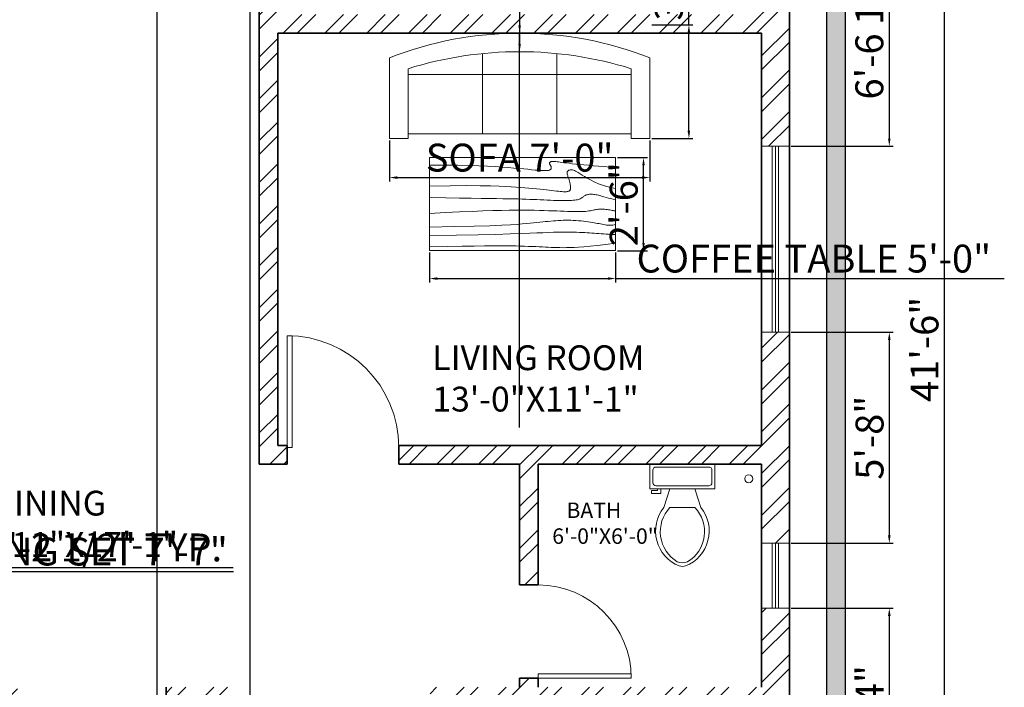
# Model space of a CAD drawing. Units: inches. Extents: x 418 to 1041, y 2094 to 2761.
# Tile 4 of 5: x 723 to 1041, y 2308 to 2523. Entities that reach past the tile are written whole.
import ezdxf

# ---------------------------------------------------------------- set-up
doc = ezdxf.new("R2010")
doc.units = ezdxf.units.IN
for name, color, linetype, lineweight in [('A-ANNO-DIMS', 2, 'Continuous', 18), ('A-AREA-IDEN', 7, 'Continuous', 18), ('A-DOOR', 4, 'Continuous', 18), ('A-FLOR-FIXT', 9, 'Continuous', 18), ('A-FURN', 8, 'Continuous', 18), ('A-GLAZ', 244, 'Continuous', 18), ('A-WALL', 7, 'Continuous', 35), ('A-WALL-PATT', 252, 'Continuous', 13), ('L-WALL', 7, 'Continuous', 25), ('L-WALL-PATT', 252, 'Continuous', 13)]:
    doc.layers.add(name, color=color, linetype=linetype, lineweight=lineweight)
doc.styles.get("Standard").update_dxf_attribs({"font": 'arial.ttf'})
doc.dimstyles.new('ISO-25', dxfattribs={"dimtxt": 9, "dimasz": 2.5, "dimexe": 1.25, "dimexo": 0.625, "dimtad": 1, "dimlunit": 3, "dimtxsty": 'Standard', "dimcen": 2.5, "dimadec": 0, "dimazin": 0, "dimtfac": 1, "dimtmove": 0, "dimatfit": 3, "dimfxl": 1, "dimarcsym": 0})

# ---------------------------------------------------------------- blocks, each defined once
blk = doc.blocks.new('*U2')
for p, q in [((0, 0), (0, -6)), ((40, 0), (40, -6))]:
    blk.add_line(p, q)
blk.add_lwpolyline([(0, 0), (0, 40), (1.75, 40), (1.75, 0)], close=True)
blk.add_arc((0, 0), 40, 0, 90)
blk = doc.blocks.new('*U7')
for p, q in [((0, 0), (0, -6)), ((-40, 0), (-40, -6))]:
    blk.add_line(p, q)
blk.add_lwpolyline([(0, 0), (0, 40), (-1.75, 40), (-1.75, 0)], close=True)
blk.add_arc((0, 0), 40, 90, 180)
blk = doc.blocks.new('*U10')
for p, q in [((9.5, -6), (9.5, -2)), ((-10, -8.5), (-8, -8.5)), ((-10, -9.5), (-10, -8.5)), ((-7, -9.5), (-10, -9.5)), ((-8, -8.5), (-8, -8)), ((-7, -8), (-7, -9.5)), ((-4, -8), (-6, -14)), ((4, -8), (6, -14)), ((4, -14), (-4, -14))]:
    blk.add_line(p, q)
blk.add_lwpolyline([(10.5, -8), (10.5, 0), (-10.5, 0), (-10.5, -8)], close=True)
for points in [[(-9.5, -2), (-9.5, -6)], [(8.5, -1), (-8.5, -1)], [(-8.5, -7), (8.5, -7)]]:
    blk.add_lwpolyline(points)
for centre, radius, start, end in [((-8.62, -1.88), 0.884, 81.8699, 188.1301), ((8.62, -1.88), 0.884, 351.8699, 98.1301), ((-8.62, -6.12), 0.884, 171.8699, 278.1301), ((8.62, -6.12), 0.884, 261.8699, 8.1301), ((3.52, -21.58), 12.17, 141.4691, 247.9714), ((4.2, -21.82), 11.33, 136.3677, 238.9468), ((-3.52, -21.58), 12.17, 292.0284, 38.5307), ((-4.2, -21.82), 11.33, 301.053, 43.6321), ((0, -27.88), 4, 245.7318, 294.2682), ((0, -29), 4, 254.8605, 285.1395)]:
    blk.add_arc(centre, radius, start, end)
blk = doc.blocks.new('Sofa - Roundback 7 ft.')
for p, q in [((-12.00002, -32.4421), (-12.00003, -6.5971)), ((11.99997, -32.4421), (11.99998, -6.5971)), ((-36.000027, -34), (-36.000027, -11.4696)), ((35.99998, -34), (35.99998, -11.4696)), ((-35.999844, -13.3819), (35.9998, -13.3819)), ((-36.000027, -32.4421), (35.99998, -32.4421))]:
    blk.add_line(p, q)
for points in [[(-36.000027, -34), (-42.000027, -34), (-42.000027, -8)], [(41.99998, -8), (41.99998, -34), (35.99998, -34)]]:
    blk.add_lwpolyline(points)
for centre, radius, start, end in [((0, -114.25), 114.25, 68.43141, 111.5686), ((-0.00001, -127.1968), 121.1968, 72.72033, 107.2797)]:
    blk.add_arc(centre, radius, start, end)
blk = doc.blocks.new('Table - Rectangular Woodgrain 60 x 30 in.')
for p, q in [((0, 0), (0, -30)), ((60, 0), (0, 0)), ((60, -30), (60, 0)), ((0, -30), (60, -30))]:
    blk.add_line(p, q)
for points in [[(0, -2.4), (4.8155, -2.418), (9.0302, -2.4688), (12.709, -2.5477), (15.9167, -2.65), (18.7181, -2.7711), (21.1781, -2.9063), (23.3616, -3.0508), (25.3333, -3.2), (27.1477, -3.3495), (28.8172, -3.4958), (30.3437, -3.636), (31.7291, -3.7667), (32.9756, -3.8849), (34.0849, -3.9875), (35.059, -4.0714), (35.9, -4.1334), (36.6114, -4.1711), (37.2041, -4.1854), (37.6906, -4.1779), (38.0833, -4.15), (38.3948, -4.1034), (38.6375, -4.0396), (38.8239, -3.9602), (38.9666, -3.8667), (39.0764, -3.7608), (39.1573, -3.6448), (39.2116, -3.521), (39.2416, -3.3917), (39.2498, -3.2593), (39.2385, -3.1261), (39.21, -2.9944), (39.1666, -2.8667), (39.111, -2.7447), (39.0468, -2.6281), (38.978, -2.5163), (38.9083, -2.4083), (38.8418, -2.3035), (38.7823, -2.201), (38.7337, -2.1001), (38.7, -2), (38.6844, -1.9003), (38.6875, -1.8021), (38.7094, -1.707), (38.75, -1.6167), (38.8094, -1.5326), (38.8875, -1.4563), (38.9844, -1.3893), (39.1, -1.3333), (39.2351, -1.2896), (39.3937, -1.2583), (39.5804, -1.2396), (39.8, -1.2333), (40.057, -1.2396), (40.3562, -1.2583), (40.7023, -1.2896), (41.1, -1.3333), (41.5547, -1.3895), (42.0755, -1.4573), (42.6721, -1.5361), (43.3542, -1.625), (44.1316, -1.7233), (45.014, -1.8302), (46.0114, -1.9449), (47.1333, -2.0667), (48.3862, -2.1947), (49.7625, -2.3281), (51.2513, -2.4663), (52.8416, -2.6083), (54.5226, -2.7535), (56.2833, -2.9011), (58.1127, -3.0501), (60, -3.2)], [(0, -9.2), (6.5759, -9.0858), (11.9385, -9.0365), (16.2527, -9.0418), (19.6833, -9.0917), (22.3952, -9.1759), (24.5531, -9.2844), (26.322, -9.4069), (27.8666, -9.5333), (29.3241, -9.6553), (30.7203, -9.7719), (32.0532, -9.8837), (33.3208, -9.9917), (34.5213, -10.0965), (35.6526, -10.199), (36.7128, -10.2999), (37.7, -10.4), (38.6129, -10.4996), (39.4531, -10.5969), (40.223, -10.6895), (40.925, -10.775), (41.5613, -10.8512), (42.1344, -10.9156), (42.6465, -10.966), (43.1, -11), (43.4976, -11.0158), (43.8437, -11.0136), (44.143, -10.9942), (44.4, -10.9583), (44.6195, -10.9069), (44.8062, -10.8406), (44.9648, -10.7603), (45.1, -10.6667), (45.2155, -10.5598), (45.3114, -10.4365), (45.3871, -10.2929), (45.4416, -10.125), (45.4743, -9.929), (45.4844, -9.7011), (45.4709, -9.4371), (45.4333, -9.1333), (45.3716, -8.7883), (45.2896, -8.4104), (45.1919, -8.0107), (45.0833, -7.6), (44.9685, -7.1893), (44.8521, -6.7896), (44.7388, -6.4117), (44.6333, -6.0667), (44.54, -5.7628), (44.4614, -5.4979), (44.4001, -5.2675), (44.3583, -5.0667), (44.3384, -4.8909), (44.3427, -4.7354), (44.3736, -4.5956), (44.4333, -4.4667), (44.5236, -4.3453), (44.6427, -4.2333), (44.7884, -4.1339), (44.9583, -4.05), (45.1501, -3.9849), (45.3614, -3.9417), (45.59, -3.9234), (45.8333, -3.9333), (46.0915, -3.9749), (46.3734, -4.0531), (46.6906, -4.1736), (47.0542, -4.3417), (47.4756, -4.5629), (47.9661, -4.8427), (48.5372, -5.1866), (49.2, -5.6), (49.9676, -6.0844), (50.8594, -6.625), (51.8965, -7.2031), (53.1, -7.8), (54.491, -8.3969), (56.0906, -8.975), (57.9199, -9.5156), (60, -10)], [(0, -12.8), (5.1847, -12.9322), (9.6213, -13.0323), (13.3963, -13.1059), (16.5958, -13.1583), (19.3063, -13.1952), (21.614, -13.2219), (23.6054, -13.2439), (25.3666, -13.2667), (26.9728, -13.2947), (28.4531, -13.3281), (29.8256, -13.3663), (31.1083, -13.4083), (32.3191, -13.4535), (33.476, -13.501), (34.597, -13.5501), (35.7, -13.6), (36.7984, -13.6497), (37.8875, -13.6979), (38.9578, -13.743), (40, -13.7833), (41.0047, -13.8174), (41.9625, -13.8438), (42.864, -13.8607), (43.7, -13.8667), (44.4631, -13.8604), (45.1552, -13.8417), (45.7801, -13.8104), (46.3416, -13.7667), (46.8439, -13.7104), (47.2906, -13.6417), (47.6858, -13.5604), (48.0333, -13.4667), (48.3375, -13.3608), (48.6042, -13.2448), (48.8396, -13.121), (49.05, -12.9917), (49.2417, -12.8593), (49.4208, -12.7261), (49.5937, -12.5944), (49.7667, -12.4667), (49.9452, -12.3451), (50.1323, -12.2313), (50.3303, -12.1268), (50.5416, -12.0333), (50.7686, -11.9524), (51.0135, -11.8854), (51.2788, -11.8341), (51.5666, -11.8), (51.8785, -11.7843), (52.2116, -11.7865), (52.562, -11.8059), (52.926, -11.8417), (53.2998, -11.8931), (53.6795, -11.9594), (54.0614, -12.0397), (54.4416, -12.1333), (54.8223, -12.2401), (55.2293, -12.3625), (55.6942, -12.5037), (56.2489, -12.6667), (56.9251, -12.8547), (57.7545, -13.0708), (58.7689, -13.3182), (60, -13.6)], [(0, -18), (5.124, -17.7273), (9.6609, -17.5057), (13.6705, -17.3303), (17.2125, -17.1958), (20.3467, -17.0973), (23.1328, -17.0297), (25.6307, -16.9878), (27.9, -16.9667), (29.9928, -16.9617), (31.9302, -16.9703), (33.7254, -16.9907), (35.3917, -17.0208), (36.9423, -17.0588), (38.3906, -17.1026), (39.7499, -17.1503), (41.0333, -17.2), (42.2519, -17.2496), (43.4073, -17.2969), (44.4986, -17.3395), (45.525, -17.375), (46.4858, -17.4012), (47.3802, -17.4156), (48.2074, -17.416), (48.9667, -17.4), (49.6583, -17.3662), (50.2872, -17.3167), (50.8595, -17.2547), (51.3812, -17.1833), (51.8584, -17.1057), (52.2971, -17.025), (52.7034, -16.9443), (53.0833, -16.8667), (53.443, -16.7951), (53.789, -16.7313), (54.128, -16.6768), (54.4666, -16.6334), (54.8115, -16.6024), (55.1693, -16.5854), (55.5465, -16.5841), (55.95, -16.6), (56.3828, -16.6337), (56.8346, -16.6823), (57.2915, -16.7418), (57.7396, -16.8084), (58.165, -16.878), (58.5539, -16.9469), (58.8924, -17.0111), (59.1666, -17.0667), (59.3679, -17.1107), (59.5078, -17.1438), (59.6032, -17.1675), (59.6708, -17.1833), (59.7275, -17.193), (59.7901, -17.1979), (59.8753, -17.1998), (60, -17.2)], [(0, -22.4), (8.0098, -22.2501), (14.4094, -22.1011), (19.4168, -21.9535), (23.25, -21.8083), (26.1269, -21.6663), (28.2656, -21.5281), (29.884, -21.3947), (31.2, -21.2667), (32.3967, -21.1448), (33.5172, -21.0292), (34.5697, -20.9198), (35.5625, -20.8167), (36.5037, -20.7198), (37.4015, -20.6292), (38.2642, -20.5448), (39.1, -20.4667), (39.9164, -20.3951), (40.7187, -20.3313), (41.5117, -20.2768), (42.3, -20.2333), (43.0883, -20.2024), (43.8812, -20.1854), (44.6836, -20.1841), (45.5, -20.2), (46.3328, -20.234), (47.1747, -20.2844), (48.0163, -20.3488), (48.8479, -20.425), (49.66, -20.5106), (50.4429, -20.6031), (51.1872, -20.7004), (51.8833, -20.8), (52.5246, -20.8999), (53.1166, -20.9995), (53.6681, -21.0983), (54.1875, -21.1958), (54.6834, -21.2919), (55.1646, -21.3859), (55.6394, -21.4777), (56.1167, -21.5667), (56.6028, -21.6515), (57.0961, -21.7266), (57.5929, -21.7852), (58.0896, -21.8208), (58.5823, -21.8268), (59.0674, -21.7964), (59.5412, -21.723), (60, -21.6)], [(0, -25.2), (8.6355, -25.0504), (15.7026, -24.9031), (21.4049, -24.7606), (25.9458, -24.625), (29.529, -24.4988), (32.3578, -24.3844), (34.6359, -24.284), (36.5667, -24.2), (38.3213, -24.1341), (39.9417, -24.0854), (41.437, -24.0523), (42.8167, -24.0333), (44.0901, -24.0268), (45.2667, -24.0313), (46.3557, -24.0451), (47.3667, -24.0667), (48.309, -24.0947), (49.1928, -24.1287), (50.0284, -24.168), (50.826, -24.2125), (51.5959, -24.2617), (52.3483, -24.3151), (53.0935, -24.3725), (53.8417, -24.4334), (54.6009, -24.497), (55.3699, -24.561), (56.1454, -24.6226), (56.9239, -24.6792), (57.7021, -24.7279), (58.4764, -24.7662), (59.2435, -24.7911), (60, -24.8)], [(0, -28.8), (5.6867, -28.6681), (10.45, -28.5698), (14.407, -28.5012), (17.675, -28.4584), (20.3711, -28.4374), (22.6125, -28.4344), (24.5164, -28.4455), (26.2, -28.4667), (27.762, -28.4947), (29.2276, -28.5281), (30.6033, -28.5663), (31.8958, -28.6084), (33.1118, -28.6535), (34.2578, -28.7011), (35.3405, -28.7501), (36.3666, -28.8), (37.3443, -28.8497), (38.288, -28.8974), (39.2137, -28.9412), (40.1375, -28.9792), (41.0753, -29.0093), (42.0432, -29.0297), (43.0572, -29.0384), (44.1333, -29.0333), (45.2936, -29.0114), (46.5843, -28.9641), (48.0579, -28.8816), (49.7666, -28.7542), (51.7629, -28.5721), (54.0989, -28.3255), (56.8272, -28.0048), (60, -27.6)]]:
    blk.add_lwpolyline(points)
blk = doc.blocks.new('*D16')
at = {"layer": 'A-ANNO-DIMS', "color": 0, "lineweight": -2, "transparency": 16777216}
for p, q in [((972.18, 2666.03), (1022.79, 2666.03)), ((1021.54, 2663.53), (1021.54, 2170.53)), ((972.18, 2168.03), (1022.79, 2168.03))]:
    blk.add_line(p, q, dxfattribs=at)
at = {"layer": 'A-ANNO-DIMS', "color": 0, "transparency": 16777216}
for points in [[(1021.13, 2663.53), (1021.96, 2663.53), (1021.54, 2666.03)], [(1021.13, 2170.53), (1021.96, 2170.53), (1021.54, 2168.03)]]:
    blk.add_solid(points, dxfattribs=at)
at = {"layer": 'Defpoints', "color": 0, "transparency": 16777216}
for p in [(971.56, 2666.03), (971.56, 2168.03), (1021.54, 2168.03)]:
    blk.add_point(p, dxfattribs=at)
at = {"layer": 'A-ANNO-DIMS', "color": 0, "transparency": 16777216, "insert": (1016.32, 2417.03), "char_height": 9, "attachment_point": 5, "rotation": 90}
blk.add_mtext('41\'-6"', dxfattribs=at)
blk = doc.blocks.new('WIN-60IN')
for p, q in [((0, 5.5), (60, 5.5)), ((0, 4.5), (60, 4.5)), ((0, 3.5), (60, 3.5))]:
    blk.add_line(p, q)
blk.add_lwpolyline([(0, 9), (60, 9), (60, 0), (0, 0)], close=True)
blk = doc.blocks.new('WIN-21IN')
for p, q in [((0, 5.5), (21, 5.5)), ((0, 4.5), (21, 4.5)), ((0, 3.5), (21, 3.5))]:
    blk.add_line(p, q)
blk.add_lwpolyline([(0, 9), (21, 9), (21, 0), (0, 0)], close=True)
blk = doc.blocks.new('*D33')
at = {"layer": 'A-ANNO-DIMS', "color": 0, "lineweight": -2, "transparency": 16777216}
for p, q in [((638.78, 2346.93), (638.78, 2347.94)), ((641.34, 2346.93), (641.34, 2347.94)), ((636.28, 2346.69), (633.78, 2346.69)), ((638.78, 2346.69), (641.34, 2346.69)), ((643.84, 2346.69), (792.12, 2346.69))]:
    blk.add_line(p, q, dxfattribs=at)
at = {"layer": 'A-ANNO-DIMS', "color": 0, "transparency": 16777216}
for points in [[(636.28, 2347.11), (636.28, 2346.28), (638.78, 2346.69)], [(643.84, 2347.11), (643.84, 2346.28), (641.34, 2346.69)]]:
    blk.add_solid(points, dxfattribs=at)
at = {"layer": 'Defpoints', "color": 0, "transparency": 16777216}
for p in [(638.78, 2346.31), (641.34, 2346.69), (641.34, 2346.31)]:
    blk.add_point(p, dxfattribs=at)
at = {"layer": 'A-ANNO-DIMS', "color": 0, "transparency": 16777216, "insert": (719.23, 2351.97), "char_height": 9, "attachment_point": 5}
blk.add_mtext('RAIL POST 0\'-2 1/2" TYP.', dxfattribs=at)
blk = doc.blocks.new('*D35')
at = {"layer": 'A-ANNO-DIMS', "color": 0, "lineweight": -2, "transparency": 16777216}
for p, q in [((598.64, 2358.4), (598.64, 2344.13)), ((689.64, 2358.4), (689.64, 2344.13)), ((601.14, 2345.38), (687.14, 2345.38)), ((689.64, 2345.38), (792.31, 2345.38))]:
    blk.add_line(p, q, dxfattribs=at)
at = {"layer": 'A-ANNO-DIMS', "color": 0, "transparency": 16777216}
for points in [[(601.14, 2345.79), (601.14, 2344.96), (598.64, 2345.38)], [(687.14, 2345.79), (687.14, 2344.96), (689.64, 2345.38)]]:
    blk.add_solid(points, dxfattribs=at)
at = {"layer": 'Defpoints', "color": 0, "transparency": 16777216}
for p in [(598.64, 2359.03), (689.64, 2359.03), (689.64, 2345.38)]:
    blk.add_point(p, dxfattribs=at)
at = {"layer": 'A-ANNO-DIMS', "color": 0, "transparency": 16777216, "insert": (742.22, 2350.65), "char_height": 9, "attachment_point": 5}
blk.add_mtext('DINING SET 7\'-7"', dxfattribs=at)
blk = doc.blocks.new('*D37')
at = {"layer": 'A-ANNO-DIMS', "color": 0, "lineweight": -2, "transparency": 16777216}
for p, q in [((842.56, 2484.4), (842.56, 2471.18)), ((926.56, 2484.4), (926.56, 2471.18)), ((845.06, 2472.43), (924.06, 2472.43))]:
    blk.add_line(p, q, dxfattribs=at)
at = {"layer": 'A-ANNO-DIMS', "color": 0, "transparency": 16777216}
for points in [[(845.06, 2472.84), (845.06, 2472.01), (842.56, 2472.43)], [(924.06, 2472.84), (924.06, 2472.01), (926.56, 2472.43)]]:
    blk.add_solid(points, dxfattribs=at)
at = {"layer": 'Defpoints', "color": 0, "transparency": 16777216}
for p in [(842.56, 2485.03), (926.56, 2485.03), (926.56, 2472.43)]:
    blk.add_point(p, dxfattribs=at)
at = {"layer": 'A-ANNO-DIMS', "color": 0, "transparency": 16777216, "insert": (884.56, 2477.71), "char_height": 9, "attachment_point": 5}
blk.add_mtext('SOFA 7\'-0"', dxfattribs=at)
blk = doc.blocks.new('*D38')
at = {"layer": 'A-ANNO-DIMS', "color": 0, "lineweight": -2, "transparency": 16777216}
for p, q in [((939.16, 2521.69), (939.16, 2570.33)), ((927.18, 2521.69), (940.41, 2521.69)), ((939.16, 2487.53), (939.16, 2519.19)), ((927.18, 2485.03), (940.41, 2485.03))]:
    blk.add_line(p, q, dxfattribs=at)
at = {"layer": 'A-ANNO-DIMS', "color": 0, "transparency": 16777216}
for points in [[(938.74, 2519.19), (939.57, 2519.19), (939.16, 2521.69)], [(938.74, 2487.53), (939.57, 2487.53), (939.16, 2485.03)]]:
    blk.add_solid(points, dxfattribs=at)
at = {"layer": 'Defpoints', "color": 0, "transparency": 16777216}
for p in [(926.56, 2521.69), (939.16, 2521.69), (926.56, 2485.03)]:
    blk.add_point(p, dxfattribs=at)
at = {"layer": 'A-ANNO-DIMS', "color": 0, "transparency": 16777216, "insert": (933.88, 2547.26), "char_height": 9, "attachment_point": 5, "rotation": 90}
blk.add_mtext('3\'-0 1/2"', dxfattribs=at)
blk = doc.blocks.new('*D39')
at = {"layer": 'A-ANNO-DIMS', "color": 0, "lineweight": -2, "transparency": 16777216}
for p, q in [((855.52, 2448.24), (855.52, 2438.61)), ((915.52, 2448.24), (915.52, 2438.61)), ((858.02, 2439.86), (913.02, 2439.86)), ((915.52, 2439.86), (1040.9, 2439.86))]:
    blk.add_line(p, q, dxfattribs=at)
at = {"layer": 'A-ANNO-DIMS', "color": 0, "transparency": 16777216}
for points in [[(858.02, 2440.28), (858.02, 2439.44), (855.52, 2439.86)], [(913.02, 2440.28), (913.02, 2439.44), (915.52, 2439.86)]]:
    blk.add_solid(points, dxfattribs=at)
at = {"layer": 'Defpoints', "color": 0, "transparency": 16777216}
for p in [(855.52, 2448.86), (915.52, 2448.86), (915.52, 2439.86)]:
    blk.add_point(p, dxfattribs=at)
at = {"layer": 'A-ANNO-DIMS', "color": 0, "transparency": 16777216, "insert": (979.46, 2445.14), "char_height": 9, "attachment_point": 5}
blk.add_mtext('COFFEE TABLE 5\'-0"', dxfattribs=at)
blk = doc.blocks.new('*D40')
at = {"layer": 'A-ANNO-DIMS', "color": 0, "lineweight": -2, "transparency": 16777216}
for p, q in [((916.15, 2478.86), (925.77, 2478.86)), ((924.52, 2451.36), (924.52, 2476.36)), ((916.15, 2448.86), (925.77, 2448.86))]:
    blk.add_line(p, q, dxfattribs=at)
at = {"layer": 'A-ANNO-DIMS', "color": 0, "transparency": 16777216}
for points in [[(924.11, 2476.36), (924.94, 2476.36), (924.52, 2478.86)], [(924.11, 2451.36), (924.94, 2451.36), (924.52, 2448.86)]]:
    blk.add_solid(points, dxfattribs=at)
at = {"layer": 'Defpoints', "color": 0, "transparency": 16777216}
for p in [(915.52, 2478.86), (924.52, 2478.86), (915.52, 2448.86)]:
    blk.add_point(p, dxfattribs=at)
at = {"layer": 'A-ANNO-DIMS', "color": 0, "transparency": 16777216, "insert": (919.3, 2463.86), "char_height": 9, "attachment_point": 5, "rotation": 90}
blk.add_mtext('2\'-6"', dxfattribs=at)
blk = doc.blocks.new('*D48')
at = {"layer": 'A-ANNO-DIMS', "color": 0, "lineweight": -2, "transparency": 16777216}
for p, q in [((972.18, 2561.03), (1005.06, 2561.03)), ((1003.81, 2558.53), (1003.81, 2485.03)), ((972.18, 2482.53), (1005.06, 2482.53))]:
    blk.add_line(p, q, dxfattribs=at)
at = {"layer": 'A-ANNO-DIMS', "color": 0, "transparency": 16777216}
for points in [[(1003.39, 2558.53), (1004.22, 2558.53), (1003.81, 2561.03)], [(1003.39, 2485.03), (1004.22, 2485.03), (1003.81, 2482.53)]]:
    blk.add_solid(points, dxfattribs=at)
at = {"layer": 'Defpoints', "color": 0, "transparency": 16777216}
for p in [(971.56, 2561.03), (971.56, 2482.53), (1003.81, 2482.53)]:
    blk.add_point(p, dxfattribs=at)
at = {"layer": 'A-ANNO-DIMS', "color": 0, "transparency": 16777216, "insert": (998.53, 2521.78), "char_height": 9, "attachment_point": 5, "rotation": 90}
blk.add_mtext('6\'-6 1/2"', dxfattribs=at)
blk = doc.blocks.new('*D49')
at = {"layer": 'A-ANNO-DIMS', "color": 0, "lineweight": -2, "transparency": 16777216}
for p, q in [((972.18, 2422.53), (1005.06, 2422.53)), ((1003.81, 2420.03), (1003.81, 2357.03)), ((972.18, 2354.53), (1005.06, 2354.53))]:
    blk.add_line(p, q, dxfattribs=at)
at = {"layer": 'A-ANNO-DIMS', "color": 0, "transparency": 16777216}
for points in [[(1003.39, 2420.03), (1004.22, 2420.03), (1003.81, 2422.53)], [(1003.39, 2357.03), (1004.22, 2357.03), (1003.81, 2354.53)]]:
    blk.add_solid(points, dxfattribs=at)
at = {"layer": 'Defpoints', "color": 0, "transparency": 16777216}
for p in [(971.56, 2422.53), (971.56, 2354.53), (1003.81, 2354.53)]:
    blk.add_point(p, dxfattribs=at)
at = {"layer": 'A-ANNO-DIMS', "color": 0, "transparency": 16777216, "insert": (998.59, 2388.53), "char_height": 9, "attachment_point": 5, "rotation": 90}
blk.add_mtext('5\'-8"', dxfattribs=at)
blk = doc.blocks.new('*D50')
at = {"layer": 'A-ANNO-DIMS', "color": 0, "lineweight": -2, "transparency": 16777216}
for p, q in [((972.18, 2333.53), (1005.06, 2333.53)), ((1003.81, 2331.03), (1003.81, 2272.26)), ((972.18, 2269.76), (1005.06, 2269.76))]:
    blk.add_line(p, q, dxfattribs=at)
at = {"layer": 'A-ANNO-DIMS', "color": 0, "transparency": 16777216}
for points in [[(1003.39, 2331.03), (1004.22, 2331.03), (1003.81, 2333.53)], [(1003.39, 2272.26), (1004.22, 2272.26), (1003.81, 2269.76)]]:
    blk.add_solid(points, dxfattribs=at)
at = {"layer": 'Defpoints', "color": 0, "transparency": 16777216}
for p in [(971.56, 2333.53), (971.56, 2269.76), (1003.81, 2269.76)]:
    blk.add_point(p, dxfattribs=at)
at = {"layer": 'A-ANNO-DIMS', "color": 0, "transparency": 16777216, "insert": (998.61, 2301.64), "char_height": 9, "attachment_point": 5, "rotation": 90}
blk.add_mtext('5\'-4"', dxfattribs=at)
blk = doc.blocks.new('*D59')
at = {"layer": 'A-ANNO-DIMS', "color": 0, "lineweight": -2, "transparency": 16777216}
for p, q in [((767.56, 2582.4), (767.56, 2100.53)), ((797.56, 2582.4), (797.56, 2100.53)), ((770.06, 2101.78), (795.06, 2101.78))]:
    blk.add_line(p, q, dxfattribs=at)
at = {"layer": 'A-ANNO-DIMS', "color": 0, "transparency": 16777216}
for points in [[(770.06, 2102.19), (770.06, 2101.36), (767.56, 2101.78)], [(795.06, 2102.19), (795.06, 2101.36), (797.56, 2101.78)]]:
    blk.add_solid(points, dxfattribs=at)
at = {"layer": 'Defpoints', "color": 0, "transparency": 16777216}
for p in [(767.56, 2583.03), (797.56, 2583.03), (797.56, 2101.78)]:
    blk.add_point(p, dxfattribs=at)
at = {"layer": 'A-ANNO-DIMS', "color": 0, "transparency": 16777216, "insert": (782.56, 2107), "char_height": 9, "attachment_point": 5}
blk.add_mtext('2\'-6"', dxfattribs=at)
blk = doc.blocks.new('*D70')
at = {"layer": 'A-ANNO-DIMS', "color": 0, "lineweight": -2, "transparency": 16777216}
for p, q in [((884.56, 2606.13), (884.56, 2515.53)), ((884.56, 2391.83), (884.56, 2513.03))]:
    blk.add_line(p, q, dxfattribs=at)
at = {"layer": 'A-ANNO-DIMS', "color": 0, "transparency": 16777216}
blk.add_solid([(884.14, 2515.53), (884.97, 2515.53), (884.56, 2513.03)], dxfattribs=at)
at = {"layer": 'Defpoints', "color": 0, "transparency": 16777216}
for p in [(884.56, 2513.03), (884.56, 2391.83)]:
    blk.add_point(p, dxfattribs=at)
at = {"layer": 'A-ANNO-DIMS', "color": 0, "transparency": 16777216, "insert": (879.34, 2585.74), "char_height": 9, "attachment_point": 5, "rotation": 90}
blk.add_mtext('R10\'-1"', dxfattribs=at)
blk = doc.blocks.new('*D71')
at = {"layer": 'A-ANNO-DIMS', "color": 0, "lineweight": -2, "transparency": 16777216}
for p, q in [((884.56, 2614.95), (884.56, 2521.53)), ((884.56, 2404.78), (884.56, 2519.03))]:
    blk.add_line(p, q, dxfattribs=at)
at = {"layer": 'A-ANNO-DIMS', "color": 0, "transparency": 16777216}
blk.add_solid([(884.14, 2521.53), (884.97, 2521.53), (884.56, 2519.03)], dxfattribs=at)
at = {"layer": 'Defpoints', "color": 0, "transparency": 16777216}
for p in [(884.56, 2519.03), (884.56, 2404.78)]:
    blk.add_point(p, dxfattribs=at)
at = {"layer": 'A-ANNO-DIMS', "color": 0, "transparency": 16777216, "insert": (879.28, 2587.58), "char_height": 9, "attachment_point": 5, "rotation": 90}
blk.add_mtext('R9\'-6 1/2"', dxfattribs=at)

msp = doc.modelspace()

# ---------------------------------------------------------------- hatches: boundary and pattern name
at = {"layer": 'A-WALL-PATT'}
h = msp.add_hatch(dxfattribs=at)
h.set_pattern_fill('ANSI32', color=256)
h.paths.add_polyline_path([(671.558, 2308.025), (554.558, 2308.025), (554.558, 2366.352), (545.558, 2366.352), (545.558, 2168.025), (555.667, 2168.025), (555.667, 2177.025), (554.558, 2177.025), (554.558, 2302.025), (671.558, 2302.025)])
h.paths.add_polyline_path([(719.558, 2299.025), (722.558, 2299.025), (722.558, 2306.225), (722.558, 2308.025), (707.558, 2308.025), (707.558, 2302.025), (710.558, 2302.025), (710.558, 2177.025), (665.344, 2177.025), (665.344, 2168.025), (719.558, 2168.025)])
h.paths.add_polyline_path([(605.344, 2177.025), (576.667, 2177.025), (576.667, 2168.025), (605.344, 2168.025)], flags=17)
h.paths.add_polyline_path([(795.654, 2308.025), (770.558, 2308.025), (770.558, 2299.025), (795.654, 2299.025)])
h.paths.add_polyline_path([(971.558, 2333.525), (962.558, 2333.525), (962.558, 2308.025), (890.558, 2308.025), (890.558, 2311.025), (886.058, 2311.025), (884.558, 2311.025), (884.558, 2308.025), (855.654, 2308.025), (855.654, 2299.025), (962.558, 2299.025), (962.558, 2269.763), (971.558, 2269.763)])
h.paths.add_polyline_path([(971.558, 2209.763), (962.558, 2209.763), (962.558, 2168.025), (971.558, 2168.025)])
h.paths.add_polyline_path([(971.558, 2422.525), (962.558, 2422.525), (962.558, 2386.025), (845.558, 2386.025), (845.558, 2380.025), (884.558, 2380.025), (884.558, 2341.025), (890.558, 2341.025), (890.558, 2380.025), (962.558, 2380.025), (962.558, 2354.525), (971.558, 2354.525)])
h.paths.add_polyline_path([(716.558, 2471.025), (651.558, 2471.025), (651.558, 2474.025), (647.058, 2474.025), (645.558, 2474.025), (645.558, 2471.025), (554.558, 2471.025), (554.558, 2484.525), (545.558, 2484.525), (545.558, 2426.352), (554.558, 2426.352), (554.558, 2465.025), (716.558, 2465.025)])
h.paths.add_polyline_path([(554.558, 2561.611), (545.558, 2561.611), (545.558, 2505.525), (554.558, 2505.525), (554.558, 2519.025), (645.558, 2519.025), (645.558, 2504.025), (651.558, 2504.025), (651.558, 2519.025), (716.558, 2519.025), (716.558, 2528.025), (710.558, 2528.025), (710.558, 2525.025), (554.558, 2525.025)])
h.paths.add_polyline_path([(971.558, 2561.025), (962.558, 2561.025), (962.558, 2525.025), (806.558, 2525.025), (806.558, 2528.025), (800.558, 2528.025), (800.558, 2380.025), (809.558, 2380.025), (809.558, 2386.025), (806.558, 2386.025), (806.558, 2519.025), (962.558, 2519.025), (962.558, 2482.525), (971.558, 2482.525)])
h.paths.add_polyline_path([(854.558, 2666.025), (769.058, 2666.025), (769.058, 2657.025), (800.558, 2657.025), (800.558, 2589.025), (797.558, 2589.025), (797.558, 2583.025), (800.558, 2583.025), (800.558, 2564.025), (806.558, 2564.025), (806.558, 2657.025), (854.558, 2657.025)])
h.paths.add_polyline_path([(971.558, 2666.025), (914.558, 2666.025), (914.558, 2657.025), (962.558, 2657.025), (962.558, 2621.025), (971.558, 2621.025)])
h.paths.add_polyline_path([(748.058, 2666.025), (662.558, 2666.025), (662.558, 2657.025), (710.558, 2657.025), (710.558, 2564.025), (716.558, 2564.025), (716.558, 2583.025), (767.558, 2583.025), (767.558, 2589.025), (716.558, 2589.025), (716.558, 2657.025), (748.058, 2657.025)])
h.paths.add_polyline_path([(602.558, 2666.025), (545.558, 2666.025), (545.558, 2621.611), (554.558, 2621.611), (554.558, 2657.025), (602.558, 2657.025)])
at = {"layer": 'L-WALL-PATT'}
h = msp.add_hatch(color=256, dxfattribs=at)
h.dxf.hatch_style = 1
h.paths.add_polyline_path([(533.558, 2678.025), (983.558, 2678.025), (983.558, 2141.025), (902.558, 2141.025), (902.558, 2168.025), (893.558, 2168.025), (893.558, 2135.025), (926.558, 2135.025), (989.558, 2135.025), (989.558, 2684.025), (527.558, 2684.025), (527.558, 2135.025), (723.29, 2135.025), (732.29, 2135.025), (732.29, 2168.025), (723.29, 2168.025), (723.29, 2141.025), (533.558, 2141.025)])

# ---------------------------------------------------------------- linework, layer by layer
at = {"layer": 'A-FLOR-FIXT'}
msp.add_circle((958.479, 2375.288), 1.303, dxfattribs=at)
at = {"layer": 'A-WALL'}
for p, q in [((971.558, 2666.025), (971.558, 2168.025)), ((800.558, 2528.025), (800.558, 2380.025)), ((806.558, 2519.025), (962.558, 2519.025)), ((806.558, 2519.025), (806.558, 2386.025)), ((962.558, 2519.025), (962.558, 2386.025)), ((806.558, 2386.025), (809.558, 2386.025)), ((809.558, 2386.025), (809.558, 2380.025)), ((845.558, 2386.025), (845.558, 2380.025)), ((845.558, 2386.025), (962.558, 2386.025)), ((800.558, 2380.025), (809.558, 2380.025)), ((845.558, 2380.025), (884.558, 2380.025)), ((884.558, 2380.025), (884.558, 2341.025)), ((890.558, 2380.025), (890.558, 2341.025)), ((890.558, 2380.025), (962.558, 2380.025)), ((962.558, 2380.025), (962.558, 2308.025)), ((884.558, 2341.025), (890.558, 2341.025)), ((884.558, 2311.025), (890.558, 2311.025)), ((884.558, 2311.025), (884.558, 2308.025)), ((890.558, 2311.025), (890.558, 2308.025)), ((770.558, 2299.025), (770.558, 2308.025))]:
    msp.add_line(p, q, dxfattribs=at)
at = {"layer": 'L-WALL'}
for p, q in [((989.558, 2684.025), (989.558, 2135.025)), ((983.558, 2678.025), (983.558, 2141.025))]:
    msp.add_line(p, q, dxfattribs=at)

# ---------------------------------------------------------------- block references
at = {"layer": 'A-DOOR', "xscale": 0.9, "yscale": 0.9, "zscale": 0.9}
msp.add_blockref('*U2', (809.558, 2385.425), dxfattribs=at)
at = {"layer": 'A-DOOR', "xscale": 0.75, "yscale": 0.75, "zscale": 0.75, "rotation": 270}
msp.add_blockref('*U7', (890.558, 2311.025), dxfattribs=at)
at = {"layer": 'A-FLOR-FIXT'}
msp.add_blockref('*U10', (937.058, 2380.025), dxfattribs=at)
at = {"layer": 'A-FURN'}
for name, p in [('Sofa - Roundback 7 ft.', (884.558, 2519.025)), ('Table - Rectangular Woodgrain 60 x 30 in.', (855.524, 2478.862))]:
    msp.add_blockref(name, p, dxfattribs=at)
at = {"layer": 'A-GLAZ'}
for name, p, rotation in [('WIN-60IN', (962.558, 2482.525), 270.0000000000008), ('WIN-21IN', (962.558, 2354.525), 270.000000000002)]:
    msp.add_blockref(name, p, dxfattribs=dict(at, rotation=rotation))

# ---------------------------------------------------------------- texts
at = {"layer": 'A-AREA-IDEN', "attachment_point": 1}
for s, width, insert, char_height in [('LIVING ROOM\\P13\'-0"X11\'-1"', 73.64672, (856.38, 2418.319), 8), ('     DINING\\P12\'-11"X17\'-1"', 69.88693, (701.72, 2371.422), 8), ('   BATH\\P6\'-0"X6\'-0"', 32.17073, (895.081, 2367.625), 5)]:
    msp.add_mtext_dynamic_manual_height_columns(s, width=width, gutter_width=12.5, heights=[0], dxfattribs=dict(at, insert=insert, char_height=char_height))

# ---------------------------------------------------------------- dimensions: what is measured, and where the dimension line sits
at = {"layer": 'A-ANNO-DIMS'}
for base, p1, p2, angle, override, picture, middle in [((1021.545, 2168.025), (971.558, 2666.025), (971.558, 2168.025), 90, {"dimclrd": 0, "dimclre": 0, "dimclrt": 0}, '*D16', (1016.325, 2417.025)), ((939.158, 2521.692), (926.558, 2485.025), (926.558, 2521.692), 90, {"dimdec": 1, "dimlfac": 1, "dimrnd": 0, "dimzin": 1, "dimdsep": 46, "dimlunit": 4, "dimfrac": 2}, '*D38', (933.876, 2547.262)), ((1003.808, 2482.525), (971.558, 2561.025), (971.558, 2482.525), 270, {"dimdec": 1, "dimlfac": 1, "dimrnd": 0, "dimzin": 1, "dimdsep": 46, "dimlunit": 4, "dimfrac": 2}, '*D48', (998.529, 2521.775)), ((924.524, 2478.862), (915.524, 2448.862), (915.524, 2478.862), 90, {"dimdec": 1, "dimlfac": 1, "dimrnd": 0, "dimzin": 1, "dimdsep": 46, "dimlunit": 4, "dimfrac": 2}, '*D40', (919.304, 2463.862)), ((1003.808, 2354.525), (971.558, 2422.525), (971.558, 2354.525), 270, {"dimdec": 1, "dimlfac": 1, "dimrnd": 0, "dimzin": 1, "dimdsep": 46, "dimlunit": 4, "dimfrac": 2}, '*D49', (998.588, 2388.525)), ((1003.808, 2269.763), (971.558, 2333.525), (971.558, 2269.763), 270, {"dimdec": 1, "dimlfac": 1, "dimrnd": 0, "dimzin": 1, "dimdsep": 46, "dimlunit": 4, "dimfrac": 2}, '*D50', (998.606, 2301.644))]:
    dim = msp.add_linear_dim(base=base, p1=p1, p2=p2, angle=angle, dimstyle='ISO-25', override=override, dxfattribs=at)
    dim.commit()
    dim.dimension.update_dxf_attribs({"geometry": picture, "text_midpoint": middle})
for center, mpoint, picture, middle in [((884.557902, 2404.775352), (884.558, 2519.025352), '*D71', (884.558, 2587.575352)), ((884.558, 2391.829), (884.558, 2513.025), '*D70', (884.558, 2585.743))]:
    dim = msp.add_radius_dim(center=center, mpoint=mpoint, dimstyle='ISO-25', override={"dimdec": 1, "dimlfac": 1, "dimrnd": 0, "dimzin": 1, "dimdsep": 46, "dimlunit": 4, "dimfrac": 2}, dxfattribs=at)
    dim.commit()
    dim.dimension.update_dxf_attribs({"geometry": picture, "text_midpoint": middle, "dimtype": 164})
dim = msp.add_linear_dim(base=(797.558, 2101.775), p1=(767.558, 2583.025), p2=(797.558, 2583.025), dimstyle='ISO-25', override={"dimdec": 1, "dimlfac": 1, "dimrnd": 0, "dimzin": 1, "dimdsep": 46, "dimlunit": 4, "dimfrac": 2}, dxfattribs=at)
dim.commit()
dim.dimension.update_dxf_attribs({"geometry": '*D59', "text_midpoint": (782.558, 2106.996)})
for base, p1, p2, text, picture, middle in [((926.558, 2472.425), (842.558, 2485.025), (926.558, 2485.025), 'SOFA <>', '*D37', (884.558, 2477.707)), ((915.524, 2439.862), (855.524, 2448.862), (915.524, 2448.862), 'COFFEE TABLE <>', '*D39', (979.464, 2445.143)), ((641.337, 2346.693), (638.777, 2346.309), (641.337, 2346.309), 'RAIL POST <> TYP.', '*D33', (719.229, 2351.974)), ((689.639, 2345.375), (598.639, 2359.025), (689.639, 2359.025), 'DINING SET <>', '*D35', (742.225, 2350.654))]:
    dim = msp.add_linear_dim(base=base, p1=p1, p2=p2, text=text, dimstyle='ISO-25', override={"dimdec": 1, "dimlfac": 1, "dimrnd": 0, "dimzin": 1, "dimdsep": 46, "dimlunit": 4, "dimfrac": 2}, dxfattribs=at)
    dim.commit()
    dim.dimension.update_dxf_attribs({"geometry": picture, "text_midpoint": middle})

doc.saveas('drawing.dxf')
